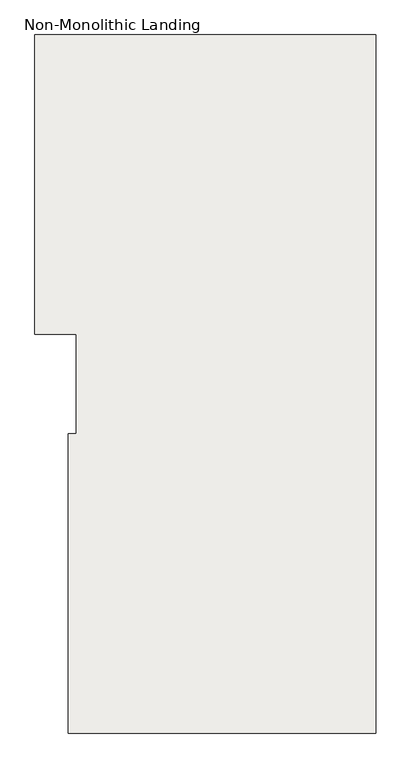
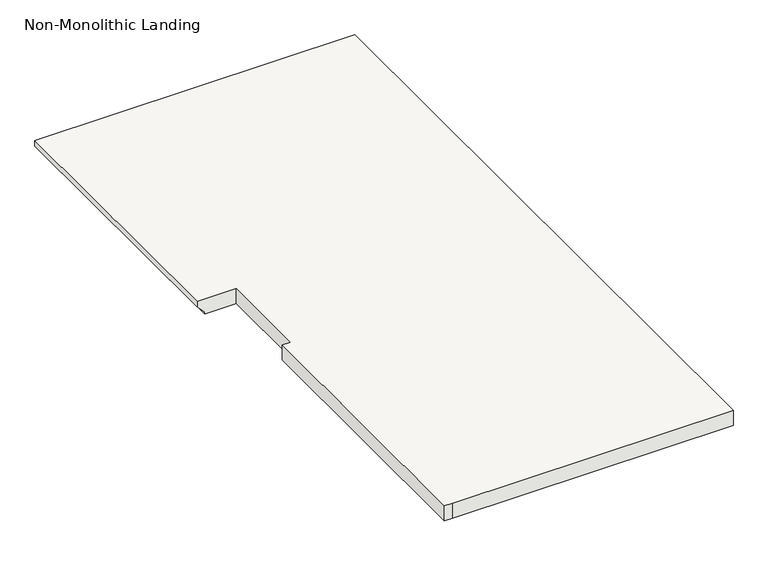
"""IFC4 building model written with IfcOpenShell, lengths in millimetres: slab geometry, Non-Monolithic Landing."""

from ifc_helpers import new_model, si_unit, origin, place, context, project, spatial, faceted_brep, source, transform, mapped, element, save


def non_monolithic_landing_28d2b2aa(model_context):
    return source(origin(), model_context, "Body", "Brep", [
        faceted_brep([(403.5869613, 2354.550634, 11089.2166667), (403.5869613, 2354.550634, 11108.2666667), (403.5869613, 3268.950634, 11108.2666667), (403.5869613, 3268.950634, 11089.2166667), (428.9869613, 2354.550634, 11063.8166667), (428.9869613, 3268.950634, 11063.8166667), (530.5869613, 2354.550634, 11108.2666667), (530.5869613, 2049.750634, 11108.2666667), (505.1869613, 2049.750634, 11108.2666667), (505.1869613, 1135.350634, 11108.2666667), (530.5869613, 1135.350634, 11108.2666667), (1444.9869613, 1135.350634, 11108.2666667), (1444.9869613, 3268.950634, 11108.2666667), (428.9869613, 2354.550634, 11057.4666667), (428.9869613, 3268.950634, 11057.4666667), (1444.9869613, 3268.950634, 11057.4666667), (1444.9869613, 1135.350634, 11057.4666667), (530.5869613, 1135.350634, 11057.4666667), (505.1869613, 1135.350634, 11057.4666667), (505.1869613, 2049.750634, 11057.4666667), (530.5869613, 2049.750634, 11057.4666667), (530.5869613, 2354.550634, 11057.4666667)], [[[0, 1, 2, 3]], [[4, 0, 3, 5]], [[6, 7, 8, 9, 10, 11, 12, 2, 1]], [[13, 14, 15, 16, 17, 18, 19, 20, 21]], [[14, 13, 4, 5]], [[6, 1, 0, 4, 13, 21]], [[7, 6, 21, 20]], [[8, 7, 20, 19]], [[9, 8, 19, 18]], [[10, 9, 18, 17]], [[11, 10, 17, 16]], [[12, 11, 16, 15]], [[2, 12, 15, 14, 5, 3]]]),
    ])


if __name__ == "__main__":
    model = new_model("IFC4")
    model_context = context("Model", 3, world=origin())
    ifc_project = project(units=[si_unit("LENGTHUNIT", "METRE", prefix="MILLI")], contexts=[model_context])
    site = spatial("IfcSite", under=ifc_project)
    building = spatial("IfcBuilding", under=site)
    placement = place(None, origin())
    non_monolithic_landing_shape = non_monolithic_landing_28d2b2aa(model_context)
    element("IfcSlab", 1, ObjectType="Non-Monolithic Landing", at=placement, inside=building, context=model_context, shape_type="MappedRepresentation", body=[
        mapped(non_monolithic_landing_shape, transform((0.0, 0.0, 0.0), x_axis=(1.0, 0.0, 0.0), y_axis=(0.0, 1.0, 0.0), z_axis=(0.0, 0.0, 1.0))),
    ])
    save(model, "model.ifc")

# Revit data of these elements
# Element 1 (IfcSlab, "Non-Monolithic Landing")
#   Materials on its faces: "BURGUNDY COLOUR"
# Materials
#   "BURGUNDY COLOUR": class "Generic", colour RGB 120 120 120, transparency 0, Cost = 0
